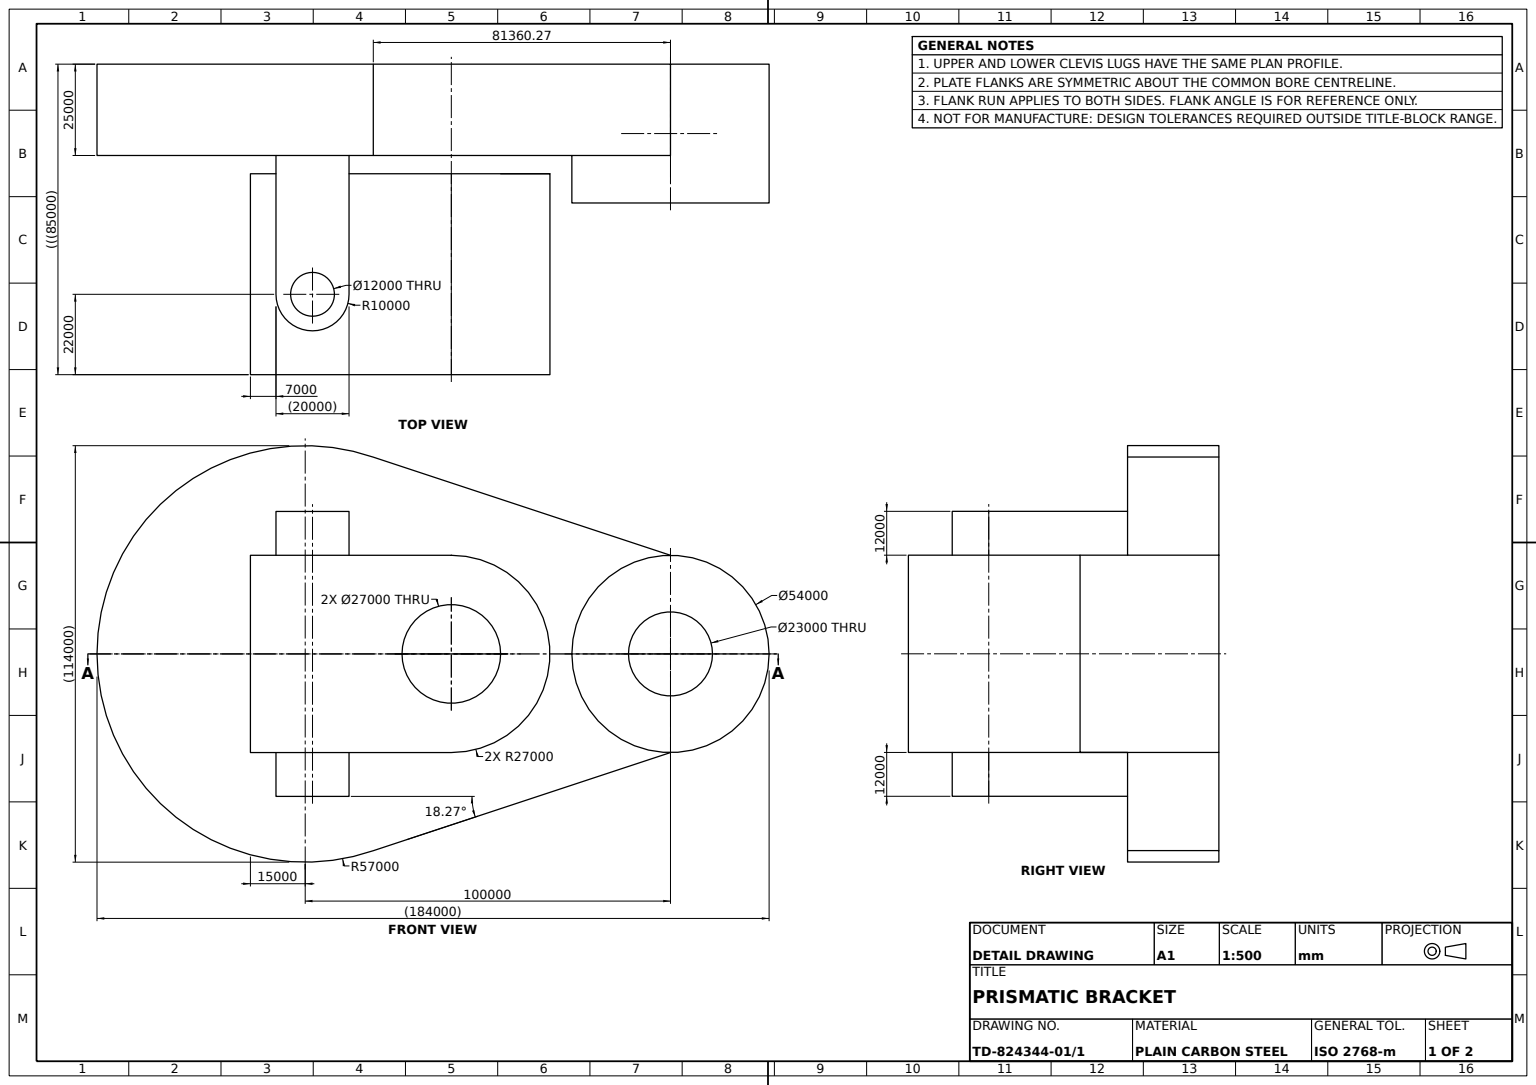
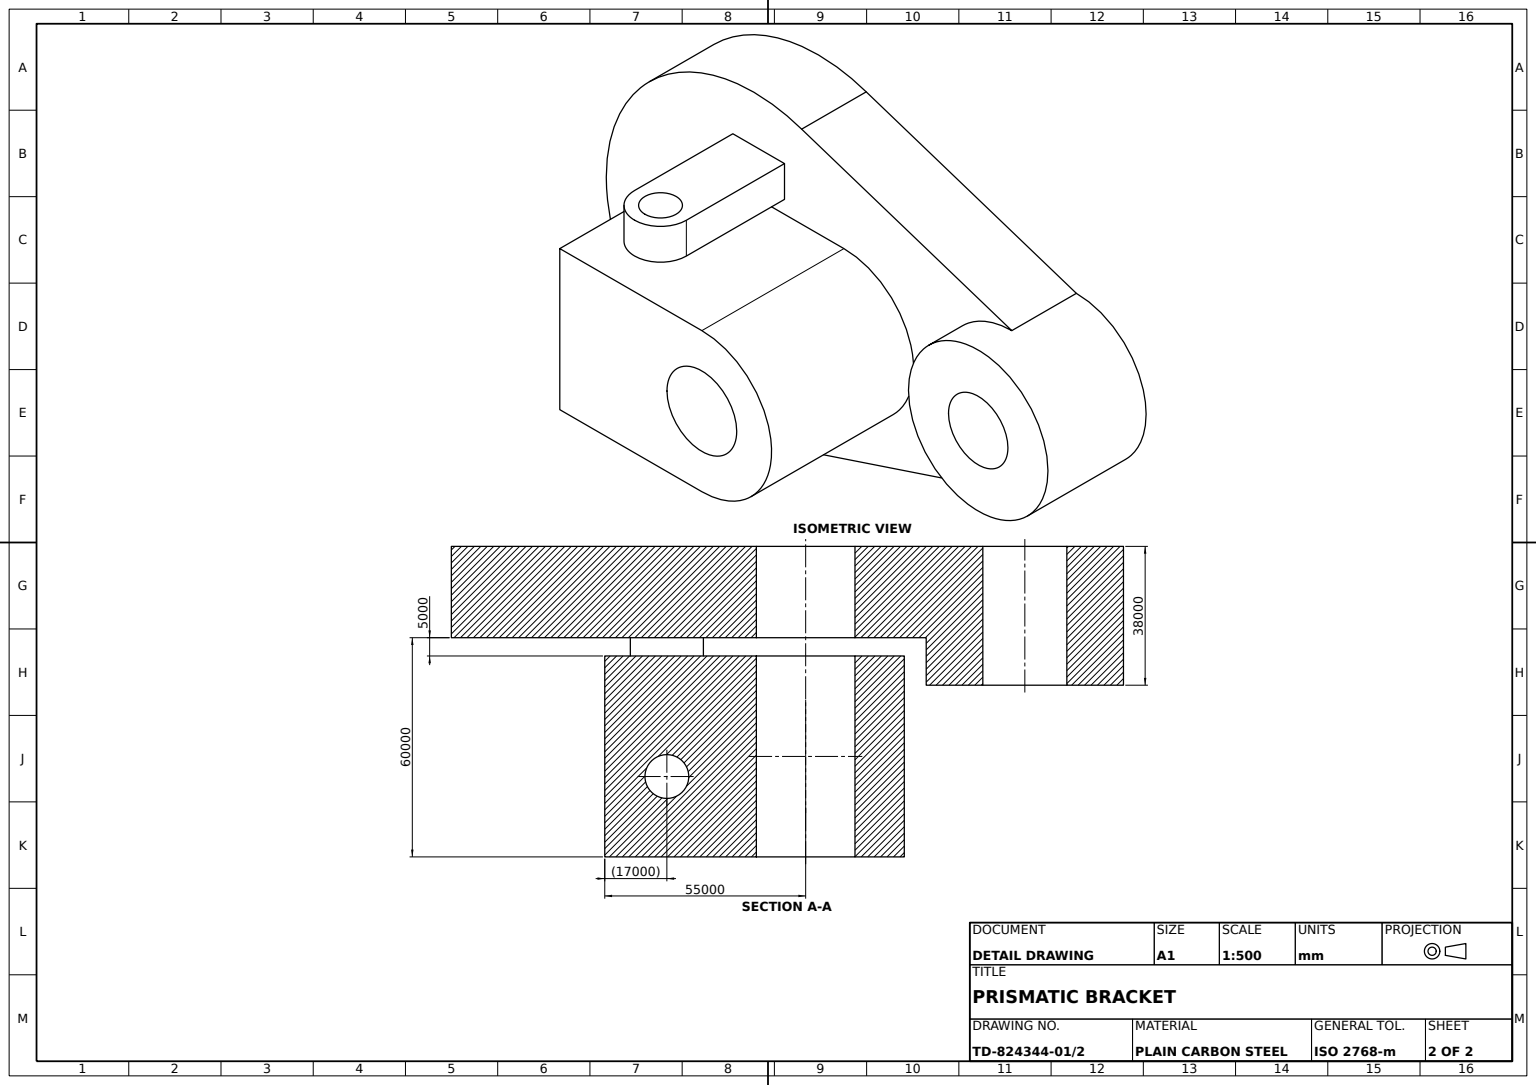
SolidWorks part; units mm, degrees
material "Plain Carbon Steel"
ref_plane "Front Plane" through (0, 0, 0) normal (0, 0, 1) x (1, 0, 0)
ref_plane "Top Plane" through (0, 0, 0) normal (0, 1, 0) x (1, 0, 0)
ref_plane "Right Plane" through (0, 0, 0) normal (1, 0, 0) x (0, 0, -1)
sketch "Hub Sketch Ø54" plane through (0, 0, 0) normal (0, 0, 1) x (1, 0, 0)
  circle A0 centre (0, 0) radius 27000
  dimension "D2" = 54000
extrude "Hub Boss Ø54" add sketch "Hub Sketch Ø54" along normal mid plane 38000
sketch "Base Plate Sketch" plane through (0, 0, 19000) normal (0, 0, 1) x (1, 0, 0)
  line L0 (0, 0) -> (100000, 0) construction
  line L1 (0, 27000) -> (81360.2668, 53866.1336)
  line L2 (0, -27000) -> (81360.2668, -53866.1336)
  arc A0 (81360.2668, -53866.1336) -> (81360.2668, 53866.1336) centre (100000, 0) ccw
  circle A1 centre (0, 0) radius 27000 construction
  arc A2 (0, -27000) -> (0, 27000) centre (0, 0) ccw
  dimension "D2" = 57000
  dimension "D1" = 100000
  dimension "D3" = 81360.2668
extrude "Base Plate" add sketch "Base Plate Sketch" against normal blind 25000
sketch "Mounting Block Sketch" plane through (0, 0, -6000) normal (0, 0, -1) x (-1, 0, 0)
  line L0 (0, 0) -> (-100000, 0) construction
  line L2 (-115000, 27000) -> (-60000, 27000)
  line L3 (-115000, 27000) -> (-115000, -27000)
  line L4 (-115000, -27000) -> (-60000, -27000)
  line L6 (-100000, 0) -> (-60000, -27000) construction
  line L7 (-100000, 0) -> (-60000, 27000) construction
  arc A0 (-60000, -27000) -> (-60000, 27000) centre (-60000, 0) ccw
  dimension "D1" = 100000
  dimension "D2" = 55000
  dimension "D3" = 15000
  dimension "D4" = 54000
  dimension "D5" = 27000
extrude "Mounting Block" add sketch "Mounting Block Sketch" along normal blind 60000
sketch "Plate Hole Sketch" plane through (0, 0, -66000) normal (0, 0, -1) x (-1, 0, 0)
  circle A0 centre (-60000, 0) radius 13500
  dimension "D1" = 27000
extrude "Plate Hole" cut sketch "Plate Hole Sketch" against normal through all
sketch "Hub Bore Sketch Ø23" plane through (0, 0, -19000) normal (0, 0, -1) x (-1, 0, 0)
  circle A0 centre (0, 0) radius 11500
  dimension "D1" = 23000
extrude "Hub Bore Ø23" cut sketch "Hub Bore Sketch Ø23" against normal through all
sketch "Block Slot Sketch" plane through (115000, 0, 0) normal (1, 0, 0) x (0, 0, -1)
  line L0 (6000, -57000) -> (6000, 57000) construction
  line L1 (6000, 27000) -> (11000, 27000)
  line L2 (6000, 27000) -> (6000, -27000)
  line L3 (6000, -27000) -> (11000, -27000)
  line L4 (11000, 27000) -> (11000, -27000)
  line L5 (6000, 27000) -> (6000, -27000) construction
  line L6 (66000, -27000) -> (6000, -27000) construction
  dimension "D1" = 5000
  dimension "D2" = 54000
extrude "Block Slot" cut sketch "Block Slot Sketch" against normal up to next
sketch "Clevis Lug 1 Sketch" plane through (0, -27000, 0) normal (0, -1, 0) x (1, 0, 0)
  line L0 (81360.2668, -6000) -> (157000, -6000) construction
  line L1 (108000, -6000) -> (88000, -6000)
  line L2 (108000, -6000) -> (108000, -44000)
  line L4 (88000, -6000) -> (88000, -44000)
  line L6 (115000, -66000) -> (115000, -11000) construction
  arc A0 (88000, -44000) -> (108000, -44000) centre (98000, -44000) ccw
  dimension "D5" = 10000
  dimension "D1" = 38000
  dimension "D2" = 20000
  dimension "D3" = 7000
  dimension "D4" = 20000
extrude "Clevis Lug 1" add sketch "Clevis Lug 1 Sketch" along normal blind 12000
sketch "Clevis Lug 2 Sketch" plane through (0, 27000, 0) normal (0, 1, 0) x (1, 0, 0)
  line L1 (108000, 6000) -> (88000, 6000)
  line L2 (108000, 6000) -> (108000, 44000)
  line L4 (88000, 6000) -> (88000, 44000)
  arc A0 (108000, 44000) -> (88000, 44000) centre (98000, 44000) ccw
  dimension "D2" = 10000
  dimension "D1" = 20000
  dimension "D3" = 38000
extrude "Clevis Lug 2" add sketch "Clevis Lug 2 Sketch" along normal blind 12000
sketch "Pin Hole Sketch Ø12" plane through (0, 39000, 0) normal (0, 1, 0) x (1, 0, 0)
  circle A0 centre (98000, 44000) radius 6000
  dimension "D1" = 12000
extrude "Pin Hole Ø12" cut sketch "Pin Hole Sketch Ø12" against normal through all
